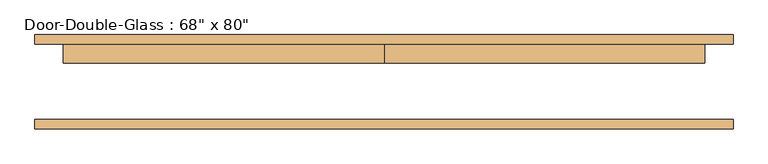
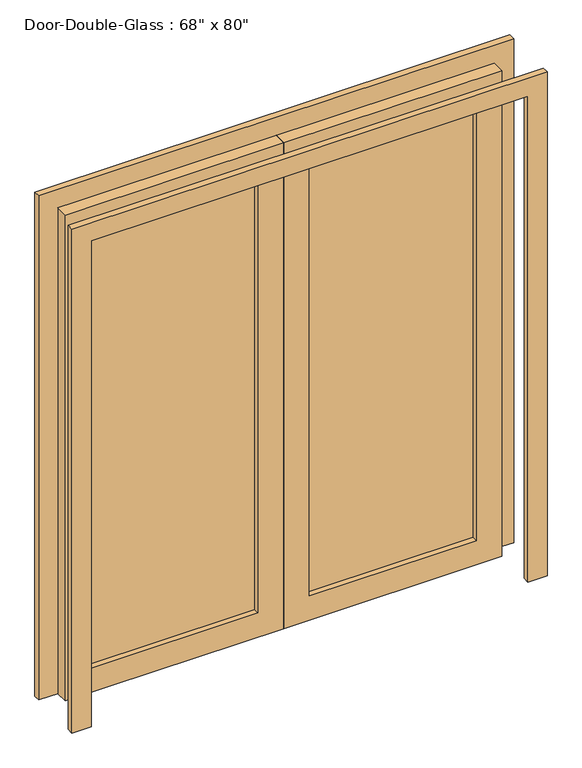
"""IFC4 building model written with IfcOpenShell, lengths in millimetres: door geometry."""

from ifc_helpers import new_model, si_unit, frame, origin, place, context, project, spatial, polyline, outline, extrude, source, transform, mapped, element, save


def door_10418eaf(model_context):
    return source(origin(), model_context, "Body", "SweptSolid", [
        extrude(outline(polyline([(2032.0, -863.6), (0.0, -863.6), (0.0, 0.0), (2032.0, 0.0), (2032.0, -863.6)]), holes=[polyline([(1930.4, -762.0), (1930.4, -101.6), (101.6, -101.6), (101.6, -762.0), (1930.4, -762.0)])]), frame((0.0, 53.18125, 0.0), z_axis=(0.0, 1.0, 0.0), x_axis=(0.0, 0.0, 1.0)), (0.0, 0.0, 1.0), 50.8),
        extrude(outline(polyline([(2032.0, 863.6), (2032.0, 0.0), (0.0, 0.0), (0.0, 863.6), (2032.0, 863.6)]), holes=[polyline([(1930.4, 762.0), (101.6, 762.0), (101.6, 101.6), (1930.4, 101.6), (1930.4, 762.0)])]), frame((0.0, 53.18125, 0.0), z_axis=(0.0, 1.0, 0.0), x_axis=(0.0, 0.0, 1.0)), (0.0, 0.0, 1.0), 50.8),
        extrude(outline(polyline([(101.6, 81.75625), (762.0, 81.75625), (762.0, 75.40625), (101.6, 75.40625), (101.6, 81.75625)])), frame((0.0, 0.0, 101.6), z_axis=(0.0, 0.0, 1.0), x_axis=(1.0, 0.0, 0.0)), (0.0, 0.0, 1.0), 1828.8),
        extrude(outline(polyline([(-762.0, 81.75625), (-101.6, 81.75625), (-101.6, 75.40625), (-762.0, 75.40625), (-762.0, 81.75625)])), frame((0.0, 0.0, 101.6), z_axis=(0.0, 0.0, 1.0), x_axis=(1.0, 0.0, 0.0)), (0.0, 0.0, 1.0), 1828.8),
        extrude(outline(polyline([(0.0, 939.8), (2108.2, 939.8), (2108.2, -939.8), (0.0, -939.8), (0.0, -863.6), (2032.0, -863.6), (2032.0, 863.6), (0.0, 863.6), (0.0, 939.8)])), frame((0.0, 103.98125, 0.0), z_axis=(0.0, 1.0, 0.0), x_axis=(0.0, 0.0, 1.0)), (0.0, 0.0, 1.0), 25.4),
        extrude(outline(polyline([(0.0, 939.8), (2108.2, 939.8), (2108.2, -939.8), (0.0, -939.8), (0.0, -863.6), (2032.0, -863.6), (2032.0, 863.6), (0.0, 863.6), (0.0, 939.8)])), frame((0.0, -124.61875, 0.0), z_axis=(0.0, 1.0, 0.0), x_axis=(0.0, 0.0, 1.0)), (0.0, 0.0, 1.0), 25.4),
    ])


if __name__ == "__main__":
    model = new_model("IFC4")
    model_context = context("Model", 3, world=origin())
    ifc_project = project(units=[si_unit("LENGTHUNIT", "METRE", prefix="MILLI")], contexts=[model_context])
    site = spatial("IfcSite", under=ifc_project)
    building = spatial("IfcBuilding", under=site)
    placement = place(None, origin())
    door_shape = door_10418eaf(model_context)
    element("IfcDoor", 1, ObjectType="Door-Double-Glass : 68\" x 80\"", at=placement, inside=building, context=model_context, shape_type="MappedRepresentation", body=[
        mapped(door_shape, transform((0.0, 0.0, 0.0), x_axis=(1.0, 0.0, 0.0), y_axis=(0.0, 1.0, 0.0), z_axis=(0.0, 0.0, 1.0))),
    ])
    save(model, "model.ifc")

# Revit data of these elements
# Type "Door-Double-Glass : 68\" x 80\""
#   Type Mark = "10"
#   Construction Type Id = "opn-d45"
#   Assembly Code = "C1020"
#   Analytic Construction = "Wood frame, double glass door "
#   W = 2' - 10"
#   Thickness = 0' - 2"
#   Thermal Resistance (R) = 1.8150 (h·ft²·°F)/BTU
#   Swing Angle [instance default] = 90.00°
#   Heat Transfer Coefficient (U) = 0.5510 BTU/(h·ft²·°F)
#   Height = 6' - 8"
#   Bottom Rail = 0' - 4"
#   Top Rail = 0' - 4"
#   Stiles = 0' - 4"
#   Trim Projection = 0' - 1"
#   Trim Width = 0' - 3"
#   Width = 5' - 8"
#   Define Thermal Properties by = 1
#   Glazing = Glass
#   Panel Material = Wood - Birch - Solid Stained Light Low Gloss
#   Trim Material = Paint - Sienna
#   Visual Light Transmittance = 0
#   Solar Heat Gain Coefficient = 0
#   Function = (empty or 0)
#   Wall Closure = (empty or 0)
# Element 1 (IfcDoor, "Door-Double-Glass : 68\" x 80\"")
#   Materials on its faces: "Wood - Birch - Solid Stained Light Low Gloss", "Paint - Sienna", "Glass"
# Materials
#   "Glass": class "Glass", colour RGB 0 128 192, transparency 0.75, Description = "Soda Lime Glass", Cost = 0
#   "Wood - Birch - Solid Stained Light Low Gloss": class "Wood", colour RGB 210 159 95, transparency 0, Cost = 0
#   "Paint - Sienna": colour RGB 118 70 51, transparency 0, Cost = 0
